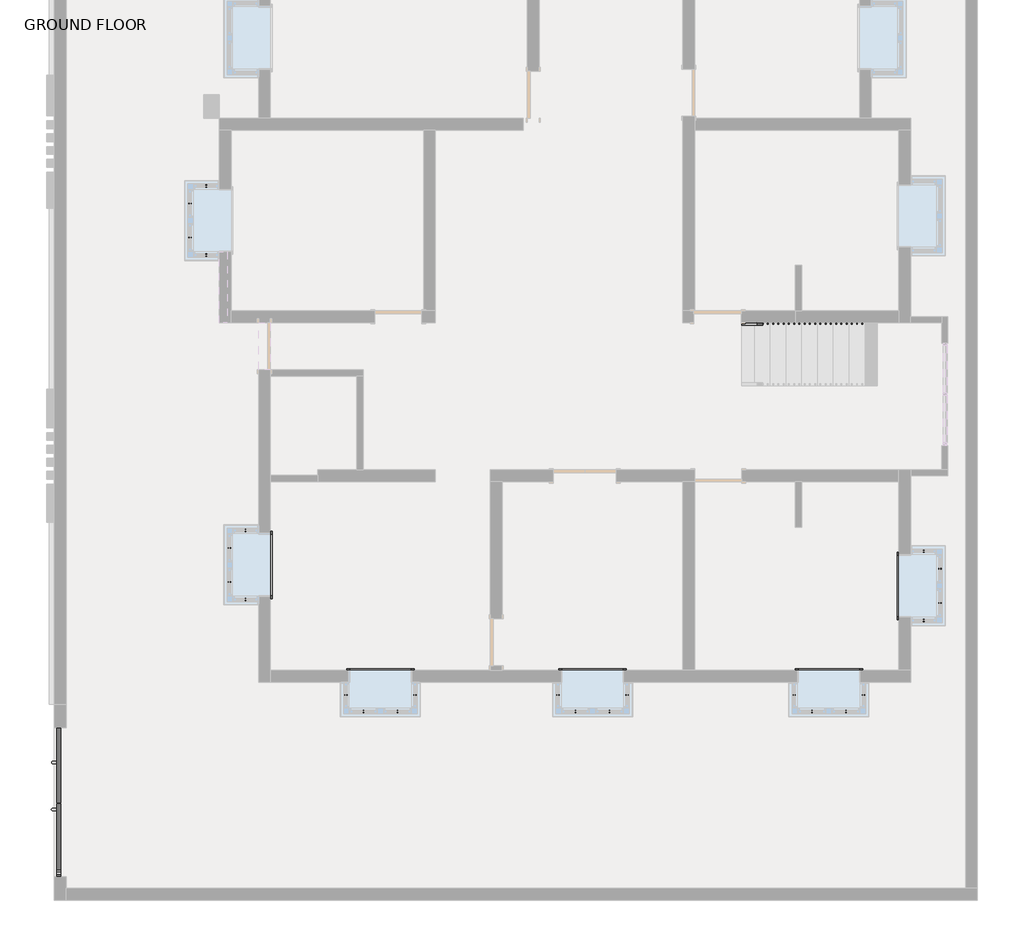
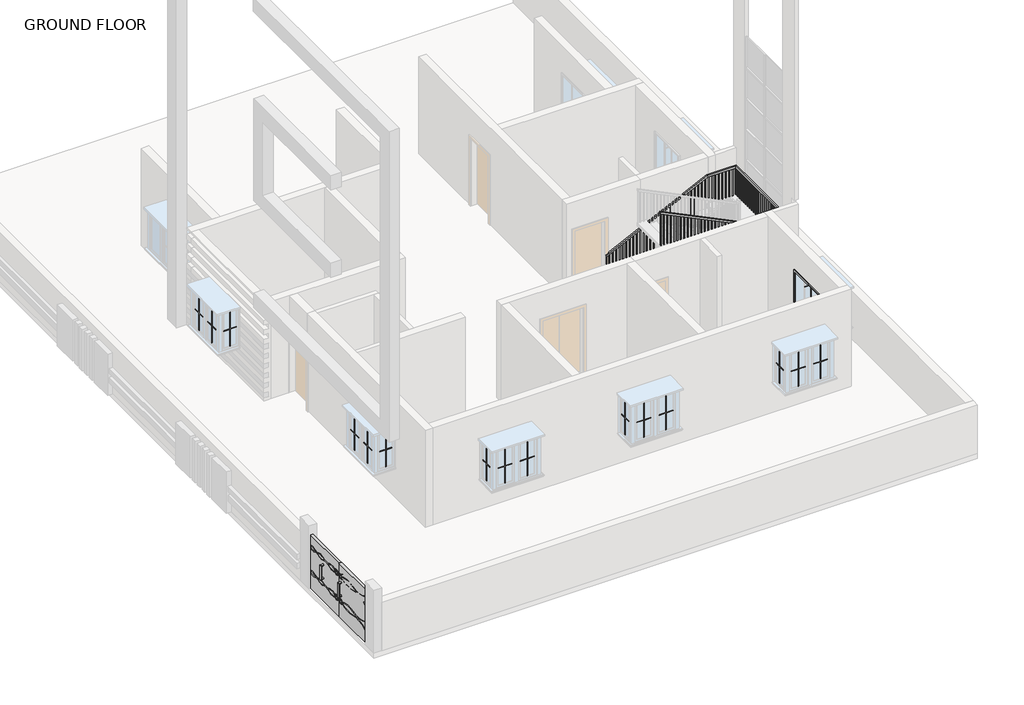
# One storey, part 4 of 5: 30 proxies, 1 railing.
"""IFC4 building model written with IfcOpenShell, lengths in millimetres."""

from ifc_helpers import new_model, si_unit, frame, origin, place, context, project, spatial, polyline, outline, extrude, faceted_brep, transform, mapped, element, save
from components import generic_models_a1fe0e04, muntin_pattern_2x2_muntin_pattern_2x2_4aee108e, muntin_pattern_2x2_muntin_pattern_2x2_f03ab90d, muntin_pattern_2x2_muntin_pattern_2x2_eb08c668, trim_window_interior_flat_picture_frame_ace0ae79

model = new_model("IFC4")

# Units and contexts
model_context = context("Model", 3, world=origin())
ifc_project = project(units=[si_unit("LENGTHUNIT", "METRE", prefix="MILLI")], contexts=[model_context])

# Site, building, storey
site = spatial("IfcSite", under=ifc_project)
building = spatial("IfcBuilding", under=site)
storey = spatial("IfcBuildingStorey", under=building, Name="GROUND FLOOR", Elevation=0.0)

# Proxies
placement = place(None, origin())
generic_models_shape = generic_models_a1fe0e04(model_context)
element("IfcBuildingElementProxy", 1, Name="Generic Models", at=placement, inside=storey, context=model_context, shape_type="MappedRepresentation", body=[
    mapped(generic_models_shape, transform((-10087.5827664, -9094.4684552, 0.0), x_axis=(0.0, -1.0, 0.0), y_axis=(1.0, 0.0, 0.0), z_axis=(0.0, 0.0, 1.0))),
])
muntin_pattern_2x2_muntin_pattern_2x2_shape = muntin_pattern_2x2_muntin_pattern_2x2_4aee108e(model_context)
element("IfcBuildingElementProxy", 2, Name="Muntin Pattern_2x2 : Muntin Pattern_2x2", ObjectType="Muntin Pattern_2x2 : Muntin Pattern_2x2", at=placement, inside=storey, context=model_context, shape_type="MappedRepresentation", body=[
    mapped(muntin_pattern_2x2_muntin_pattern_2x2_shape, transform((-7576.6665084, 1871.733346, 1035.05), x_axis=(0.0, 1.0, 0.0), y_axis=(-1.0, 0.0, 0.0), z_axis=(0.0, 0.0, 1.0))),
])
element("IfcBuildingElementProxy", 3, Name="Muntin Pattern_2x2 : Muntin Pattern_2x2", ObjectType="Muntin Pattern_2x2 : Muntin Pattern_2x2", at=placement, inside=storey, context=model_context, shape_type="MappedRepresentation", body=[
    mapped(muntin_pattern_2x2_muntin_pattern_2x2_shape, transform((-3553.9415084, -7319.891654, 1035.05), x_axis=(-1.0, 0.0, 0.0), y_axis=(0.0, -1.0, 0.0), z_axis=(0.0, 0.0, 1.0))),
])
element("IfcBuildingElementProxy", 4, Name="Muntin Pattern_2x2 : Muntin Pattern_2x2", ObjectType="Muntin Pattern_2x2 : Muntin Pattern_2x2", at=placement, inside=storey, context=model_context, shape_type="MappedRepresentation", body=[
    mapped(muntin_pattern_2x2_muntin_pattern_2x2_shape, transform((5145.5584916, -7319.891654, 1035.05), x_axis=(-1.0, 0.0, 0.0), y_axis=(0.0, -1.0, 0.0), z_axis=(0.0, 0.0, 1.0))),
])
element("IfcBuildingElementProxy", 5, Name="Muntin Pattern_2x2 : Muntin Pattern_2x2", ObjectType="Muntin Pattern_2x2 : Muntin Pattern_2x2", at=placement, inside=storey, context=model_context, shape_type="MappedRepresentation", body=[
    mapped(muntin_pattern_2x2_muntin_pattern_2x2_shape, transform((560.8584916, -7319.891654, 1035.05), x_axis=(-1.0, 0.0, 0.0), y_axis=(0.0, -1.0, 0.0), z_axis=(0.0, 0.0, 1.0))),
])
element("IfcBuildingElementProxy", 6, Name="Muntin Pattern_2x2 : Muntin Pattern_2x2", ObjectType="Muntin Pattern_2x2 : Muntin Pattern_2x2", at=placement, inside=storey, context=model_context, shape_type="MappedRepresentation", body=[
    mapped(muntin_pattern_2x2_muntin_pattern_2x2_shape, transform((-6814.6665084, -4808.466654, 1035.05), x_axis=(0.0, 1.0, 0.0), y_axis=(-1.0, 0.0, 0.0), z_axis=(0.0, 0.0, 1.0))),
])
element("IfcBuildingElementProxy", 7, Name="Muntin Pattern_2x2 : Muntin Pattern_2x2", ObjectType="Muntin Pattern_2x2 : Muntin Pattern_2x2", at=placement, inside=storey, context=model_context, shape_type="MappedRepresentation", body=[
    mapped(muntin_pattern_2x2_muntin_pattern_2x2_shape, transform((6971.1834916, -4554.466654, 1035.05), x_axis=(0.0, -1.0, 0.0), y_axis=(1.0, 0.0, 0.0), z_axis=(0.0, 0.0, 1.0))),
])
muntin_pattern_2x2_muntin_pattern_2x2_2_shape = muntin_pattern_2x2_muntin_pattern_2x2_f03ab90d(model_context)
element("IfcBuildingElementProxy", 8, Name="Muntin Pattern_2x2 : Muntin Pattern_2x2", ObjectType="Muntin Pattern_2x2 : Muntin Pattern_2x2", at=placement, inside=storey, context=model_context, shape_type="MappedRepresentation", body=[
    mapped(muntin_pattern_2x2_muntin_pattern_2x2_2_shape, transform((-7262.3415084, 1532.008346, 1035.05), x_axis=(1.0, 0.0, 0.0), y_axis=(0.0, 1.0, 0.0), z_axis=(0.0, 0.0, 1.0))),
])
element("IfcBuildingElementProxy", 9, Name="Muntin Pattern_2x2 : Muntin Pattern_2x2", ObjectType="Muntin Pattern_2x2 : Muntin Pattern_2x2", at=placement, inside=storey, context=model_context, shape_type="MappedRepresentation", body=[
    mapped(muntin_pattern_2x2_muntin_pattern_2x2_2_shape, transform((-7262.3415084, 2871.858346, 1035.05), x_axis=(-1.0, 0.0, 0.0), y_axis=(0.0, -1.0, 0.0), z_axis=(0.0, 0.0, 1.0))),
])
element("IfcBuildingElementProxy", 10, Name="Muntin Pattern_2x2 : Muntin Pattern_2x2", ObjectType="Muntin Pattern_2x2 : Muntin Pattern_2x2", at=placement, inside=storey, context=model_context, shape_type="MappedRepresentation", body=[
    mapped(muntin_pattern_2x2_muntin_pattern_2x2_2_shape, transform((-3214.2165084, -7005.566654, 1035.05), x_axis=(0.0, 1.0, 0.0), y_axis=(-1.0, 0.0, 0.0), z_axis=(0.0, 0.0, 1.0))),
])
element("IfcBuildingElementProxy", 11, Name="Muntin Pattern_2x2 : Muntin Pattern_2x2", ObjectType="Muntin Pattern_2x2 : Muntin Pattern_2x2", at=placement, inside=storey, context=model_context, shape_type="MappedRepresentation", body=[
    mapped(muntin_pattern_2x2_muntin_pattern_2x2_2_shape, transform((-4554.0665084, -7005.566654, 1035.05), x_axis=(0.0, -1.0, 0.0), y_axis=(1.0, 0.0, 0.0), z_axis=(0.0, 0.0, 1.0))),
])
element("IfcBuildingElementProxy", 12, Name="Muntin Pattern_2x2 : Muntin Pattern_2x2", ObjectType="Muntin Pattern_2x2 : Muntin Pattern_2x2", at=placement, inside=storey, context=model_context, shape_type="MappedRepresentation", body=[
    mapped(muntin_pattern_2x2_muntin_pattern_2x2_2_shape, transform((5485.2834916, -7005.566654, 1035.05), x_axis=(0.0, 1.0, 0.0), y_axis=(-1.0, 0.0, 0.0), z_axis=(0.0, 0.0, 1.0))),
])
element("IfcBuildingElementProxy", 13, Name="Muntin Pattern_2x2 : Muntin Pattern_2x2", ObjectType="Muntin Pattern_2x2 : Muntin Pattern_2x2", at=placement, inside=storey, context=model_context, shape_type="MappedRepresentation", body=[
    mapped(muntin_pattern_2x2_muntin_pattern_2x2_2_shape, transform((4145.4334916, -7005.566654, 1035.05), x_axis=(0.0, -1.0, 0.0), y_axis=(1.0, 0.0, 0.0), z_axis=(0.0, 0.0, 1.0))),
])
element("IfcBuildingElementProxy", 14, Name="Muntin Pattern_2x2 : Muntin Pattern_2x2", ObjectType="Muntin Pattern_2x2 : Muntin Pattern_2x2", at=placement, inside=storey, context=model_context, shape_type="MappedRepresentation", body=[
    mapped(muntin_pattern_2x2_muntin_pattern_2x2_2_shape, transform((900.5834916, -7005.566654, 1035.05), x_axis=(0.0, 1.0, 0.0), y_axis=(-1.0, 0.0, 0.0), z_axis=(0.0, 0.0, 1.0))),
])
element("IfcBuildingElementProxy", 15, Name="Muntin Pattern_2x2 : Muntin Pattern_2x2", ObjectType="Muntin Pattern_2x2 : Muntin Pattern_2x2", at=placement, inside=storey, context=model_context, shape_type="MappedRepresentation", body=[
    mapped(muntin_pattern_2x2_muntin_pattern_2x2_2_shape, transform((-439.2665084, -7005.566654, 1035.05), x_axis=(0.0, -1.0, 0.0), y_axis=(1.0, 0.0, 0.0), z_axis=(0.0, 0.0, 1.0))),
])
element("IfcBuildingElementProxy", 16, Name="Muntin Pattern_2x2 : Muntin Pattern_2x2", ObjectType="Muntin Pattern_2x2 : Muntin Pattern_2x2", at=placement, inside=storey, context=model_context, shape_type="MappedRepresentation", body=[
    mapped(muntin_pattern_2x2_muntin_pattern_2x2_2_shape, transform((-6500.3415084, -5148.191654, 1035.05), x_axis=(1.0, 0.0, 0.0), y_axis=(0.0, 1.0, 0.0), z_axis=(0.0, 0.0, 1.0))),
])
element("IfcBuildingElementProxy", 17, Name="Muntin Pattern_2x2 : Muntin Pattern_2x2", ObjectType="Muntin Pattern_2x2 : Muntin Pattern_2x2", at=placement, inside=storey, context=model_context, shape_type="MappedRepresentation", body=[
    mapped(muntin_pattern_2x2_muntin_pattern_2x2_2_shape, transform((-6500.3415084, -3808.341654, 1035.05), x_axis=(-1.0, 0.0, 0.0), y_axis=(0.0, -1.0, 0.0), z_axis=(0.0, 0.0, 1.0))),
])
element("IfcBuildingElementProxy", 18, Name="Muntin Pattern_2x2 : Muntin Pattern_2x2", ObjectType="Muntin Pattern_2x2 : Muntin Pattern_2x2", at=placement, inside=storey, context=model_context, shape_type="MappedRepresentation", body=[
    mapped(muntin_pattern_2x2_muntin_pattern_2x2_2_shape, transform((6656.8584916, -4214.741654, 1035.05), x_axis=(-1.0, 0.0, 0.0), y_axis=(0.0, -1.0, 0.0), z_axis=(0.0, 0.0, 1.0))),
])
element("IfcBuildingElementProxy", 19, Name="Muntin Pattern_2x2 : Muntin Pattern_2x2", ObjectType="Muntin Pattern_2x2 : Muntin Pattern_2x2", at=placement, inside=storey, context=model_context, shape_type="MappedRepresentation", body=[
    mapped(muntin_pattern_2x2_muntin_pattern_2x2_2_shape, transform((6656.8584916, -5554.591654, 1035.05), x_axis=(1.0, 0.0, 0.0), y_axis=(0.0, 1.0, 0.0), z_axis=(0.0, 0.0, 1.0))),
])
muntin_pattern_2x2_muntin_pattern_2x2_3_shape = muntin_pattern_2x2_muntin_pattern_2x2_eb08c668(model_context)
element("IfcBuildingElementProxy", 20, Name="Muntin Pattern_2x2 : Muntin Pattern_2x2", ObjectType="Muntin Pattern_2x2 : Muntin Pattern_2x2", at=placement, inside=storey, context=model_context, shape_type="MappedRepresentation", body=[
    mapped(muntin_pattern_2x2_muntin_pattern_2x2_3_shape, transform((-7576.6665084, 2532.133346, 1035.05), x_axis=(0.0, -1.0, 0.0), y_axis=(1.0, 0.0, 0.0), z_axis=(0.0, 0.0, 1.0))),
])
element("IfcBuildingElementProxy", 21, Name="Muntin Pattern_2x2 : Muntin Pattern_2x2", ObjectType="Muntin Pattern_2x2 : Muntin Pattern_2x2", at=placement, inside=storey, context=model_context, shape_type="MappedRepresentation", body=[
    mapped(muntin_pattern_2x2_muntin_pattern_2x2_3_shape, transform((-4214.3415084, -7319.891654, 1035.05), x_axis=(1.0, 0.0, 0.0), y_axis=(0.0, 1.0, 0.0), z_axis=(0.0, 0.0, 1.0))),
])
element("IfcBuildingElementProxy", 22, Name="Muntin Pattern_2x2 : Muntin Pattern_2x2", ObjectType="Muntin Pattern_2x2 : Muntin Pattern_2x2", at=placement, inside=storey, context=model_context, shape_type="MappedRepresentation", body=[
    mapped(muntin_pattern_2x2_muntin_pattern_2x2_3_shape, transform((4485.1584916, -7319.891654, 1035.05), x_axis=(1.0, 0.0, 0.0), y_axis=(0.0, 1.0, 0.0), z_axis=(0.0, 0.0, 1.0))),
])
element("IfcBuildingElementProxy", 23, Name="Muntin Pattern_2x2 : Muntin Pattern_2x2", ObjectType="Muntin Pattern_2x2 : Muntin Pattern_2x2", at=placement, inside=storey, context=model_context, shape_type="MappedRepresentation", body=[
    mapped(muntin_pattern_2x2_muntin_pattern_2x2_3_shape, transform((-99.5415084, -7319.891654, 1035.05), x_axis=(1.0, 0.0, 0.0), y_axis=(0.0, 1.0, 0.0), z_axis=(0.0, 0.0, 1.0))),
])
element("IfcBuildingElementProxy", 24, Name="Muntin Pattern_2x2 : Muntin Pattern_2x2", ObjectType="Muntin Pattern_2x2 : Muntin Pattern_2x2", at=placement, inside=storey, context=model_context, shape_type="MappedRepresentation", body=[
    mapped(muntin_pattern_2x2_muntin_pattern_2x2_3_shape, transform((-6814.6665084, -4148.066654, 1035.05), x_axis=(0.0, -1.0, 0.0), y_axis=(1.0, 0.0, 0.0), z_axis=(0.0, 0.0, 1.0))),
])
element("IfcBuildingElementProxy", 25, Name="Muntin Pattern_2x2 : Muntin Pattern_2x2", ObjectType="Muntin Pattern_2x2 : Muntin Pattern_2x2", at=placement, inside=storey, context=model_context, shape_type="MappedRepresentation", body=[
    mapped(muntin_pattern_2x2_muntin_pattern_2x2_3_shape, transform((6971.1834916, -5214.866654, 1035.05), x_axis=(0.0, 1.0, 0.0), y_axis=(-1.0, 0.0, 0.0), z_axis=(0.0, 0.0, 1.0))),
])
trim_window_interior_flat_picture_frame_shape = trim_window_interior_flat_picture_frame_ace0ae79(model_context)
element("IfcBuildingElementProxy", 26, Name="Trim-Window-Interior-Flat : Picture Frame", ObjectType="Trim-Window-Interior-Flat : Picture Frame", at=placement, inside=storey, context=model_context, shape_type="MappedRepresentation", body=[
    mapped(trim_window_interior_flat_picture_frame_shape, transform((-3884.1415084, -6522.966654, 2184.4), x_axis=(-1.0, 0.0, 0.0), y_axis=(0.0, 0.0, 1.0), z_axis=(0.0, 1.0, 0.0))),
])
element("IfcBuildingElementProxy", 27, Name="Trim-Window-Interior-Flat : Picture Frame", ObjectType="Trim-Window-Interior-Flat : Picture Frame", at=placement, inside=storey, context=model_context, shape_type="MappedRepresentation", body=[
    mapped(trim_window_interior_flat_picture_frame_shape, transform((4815.3584916, -6522.966654, 2184.4), x_axis=(-1.0, 0.0, 0.0), y_axis=(0.0, 0.0, 1.0), z_axis=(0.0, 1.0, 0.0))),
])
element("IfcBuildingElementProxy", 28, Name="Trim-Window-Interior-Flat : Picture Frame", ObjectType="Trim-Window-Interior-Flat : Picture Frame", at=placement, inside=storey, context=model_context, shape_type="MappedRepresentation", body=[
    mapped(trim_window_interior_flat_picture_frame_shape, transform((230.6584916, -6522.966654, 2184.4), x_axis=(-1.0, 0.0, 0.0), y_axis=(0.0, 0.0, 1.0), z_axis=(0.0, 1.0, 0.0))),
])
element("IfcBuildingElementProxy", 29, Name="Trim-Window-Interior-Flat : Picture Frame", ObjectType="Trim-Window-Interior-Flat : Picture Frame", at=placement, inside=storey, context=model_context, shape_type="MappedRepresentation", body=[
    mapped(trim_window_interior_flat_picture_frame_shape, transform((-6017.7415084, -4478.266654, 2184.4), x_axis=(0.0, 1.0, 0.0), y_axis=(0.0, 0.0, 1.0), z_axis=(1.0, 0.0, 0.0))),
])
element("IfcBuildingElementProxy", 30, Name="Trim-Window-Interior-Flat : Picture Frame", ObjectType="Trim-Window-Interior-Flat : Picture Frame", at=placement, inside=storey, context=model_context, shape_type="MappedRepresentation", body=[
    mapped(trim_window_interior_flat_picture_frame_shape, transform((6174.2584916, -4884.666654, 2184.4), x_axis=(0.0, -1.0, 0.0), y_axis=(0.0, 0.0, 1.0), z_axis=(-1.0, 0.0, 0.0))),
])

# Railing
element("IfcRailing", 31, ObjectType="Handrail - Rectangular", at=placement, inside=storey, context=model_context, shape_type="SolidModel", body=[
    faceted_brep([(3126.2584916, 220.733346, 1059.8727273), (3126.2584916, 220.733346, 1003.3956113), (3126.2584916, 169.933346, 1003.3956113), (3126.2584916, 169.933346, 1059.8727273), (6120.7829507, 220.733346, 2514.6), (6132.4691705, 220.733346, 2463.8), (6132.4691705, 169.933346, 2463.8), (6120.7829507, 169.933346, 2514.6), (7009.1350459, 220.733346, 2514.6), (7009.1350459, 220.733346, 2463.8), (6958.3350459, 169.933346, 2463.8), (6958.3350459, 169.933346, 2514.6), (7009.1350459, -2636.766654, 2514.6), (7009.1350459, -2636.766654, 2463.8), (6958.3350459, -2585.966654, 2463.8), (6958.3350459, -2585.966654, 2514.6), (6420.2353966, -2636.766654, 2514.6), (6408.5491768, -2636.766654, 2463.8), (6408.5491768, -2585.966654, 2463.8), (6420.2353966, -2585.966654, 2514.6), (3126.2584916, -2636.766654, 4114.8), (3126.2584916, -2585.966654, 4114.8), (3126.2584916, -2585.966654, 4058.322884), (3126.2584916, -2636.766654, 4058.322884)], [[[0, 1, 2, 3]], [[1, 0, 4, 5]], [[2, 1, 5, 6]], [[3, 2, 6, 7]], [[0, 3, 7, 4]], [[5, 4, 8, 9]], [[6, 5, 9, 10]], [[7, 6, 10, 11]], [[4, 7, 11, 8]], [[9, 8, 12, 13]], [[10, 9, 13, 14]], [[11, 10, 14, 15]], [[8, 11, 15, 12]], [[13, 12, 16, 17]], [[14, 13, 17, 18]], [[15, 14, 18, 19]], [[12, 15, 19, 16]], [[20, 21, 22, 23]], [[17, 16, 20, 23]], [[18, 17, 23, 22]], [[19, 18, 22, 21]], [[16, 19, 21, 20]]]),
    extrude(outline(polyline([(4015.2077556, 3215.0100459), (3054.9272727, 3215.0100459), (3054.9272727, 3234.0600459), (4005.9533465, 3234.0600459), (4015.2077556, 3215.0100459)])), frame((0.0, -2620.891654, 0.0), z_axis=(0.0, 1.0, 0.0), x_axis=(0.0, 0.0, 1.0)), (0.0, 0.0, 1.0), 19.05),
    extrude(outline(polyline([(3965.8509068, 3316.6100459), (3054.9272727, 3316.6100459), (3054.9272727, 3335.6600459), (3956.5964977, 3335.6600459), (3965.8509068, 3316.6100459)])), frame((0.0, -2620.891654, 0.0), z_axis=(0.0, 1.0, 0.0), x_axis=(0.0, 0.0, 1.0)), (0.0, 0.0, 1.0), 19.05),
    extrude(outline(polyline([(3916.494058, 3418.2100459), (2909.4545455, 3418.2100459), (2909.4545455, 3437.2600459), (3907.2396489, 3437.2600459), (3916.494058, 3418.2100459)])), frame((0.0, -2620.891654, 0.0), z_axis=(0.0, 1.0, 0.0), x_axis=(0.0, 0.0, 1.0)), (0.0, 0.0, 1.0), 19.05),
    extrude(outline(polyline([(3867.1372093, 3519.8100459), (2909.4545455, 3519.8100459), (2909.4545455, 3538.8600459), (3857.8828001, 3538.8600459), (3867.1372093, 3519.8100459)])), frame((0.0, -2620.891654, 0.0), z_axis=(0.0, 1.0, 0.0), x_axis=(0.0, 0.0, 1.0)), (0.0, 0.0, 1.0), 19.05),
    extrude(outline(polyline([(3817.7803605, 3621.4100459), (2909.4545455, 3621.4100459), (2909.4545455, 3640.4600459), (3808.5259513, 3640.4600459), (3817.7803605, 3621.4100459)])), frame((0.0, -2620.891654, 0.0), z_axis=(0.0, 1.0, 0.0), x_axis=(0.0, 0.0, 1.0)), (0.0, 0.0, 1.0), 19.05),
    extrude(outline(polyline([(3768.4235117, 3723.0100459), (2763.9818182, 3723.0100459), (2763.9818182, 3742.0600459), (3759.1691025, 3742.0600459), (3768.4235117, 3723.0100459)])), frame((0.0, -2620.891654, 0.0), z_axis=(0.0, 1.0, 0.0), x_axis=(0.0, 0.0, 1.0)), (0.0, 0.0, 1.0), 19.05),
    extrude(outline(polyline([(3719.0666629, 3824.6100459), (2763.9818182, 3824.6100459), (2763.9818182, 3843.6600459), (3709.8122538, 3843.6600459), (3719.0666629, 3824.6100459)])), frame((0.0, -2620.891654, 0.0), z_axis=(0.0, 1.0, 0.0), x_axis=(0.0, 0.0, 1.0)), (0.0, 0.0, 1.0), 19.05),
    extrude(outline(polyline([(3669.7098141, 3926.2100459), (2763.9818182, 3926.2100459), (2763.9818182, 3945.2600459), (3660.455405, 3945.2600459), (3669.7098141, 3926.2100459)])), frame((0.0, -2620.891654, 0.0), z_axis=(0.0, 1.0, 0.0), x_axis=(0.0, 0.0, 1.0)), (0.0, 0.0, 1.0), 19.05),
    extrude(outline(polyline([(3620.3529653, 4027.8100459), (2618.5090909, 4027.8100459), (2618.5090909, 4046.8600459), (3611.0985562, 4046.8600459), (3620.3529653, 4027.8100459)])), frame((0.0, -2620.891654, 0.0), z_axis=(0.0, 1.0, 0.0), x_axis=(0.0, 0.0, 1.0)), (0.0, 0.0, 1.0), 19.05),
    extrude(outline(polyline([(3570.9961165, 4129.4100459), (2618.5090909, 4129.4100459), (2618.5090909, 4148.4600459), (3561.7417074, 4148.4600459), (3570.9961165, 4129.4100459)])), frame((0.0, -2620.891654, 0.0), z_axis=(0.0, 1.0, 0.0), x_axis=(0.0, 0.0, 1.0)), (0.0, 0.0, 1.0), 19.05),
    extrude(outline(polyline([(3521.6392678, 4231.0100459), (2618.5090909, 4231.0100459), (2618.5090909, 4250.0600459), (3512.3848586, 4250.0600459), (3521.6392678, 4231.0100459)])), frame((0.0, -2620.891654, 0.0), z_axis=(0.0, 1.0, 0.0), x_axis=(0.0, 0.0, 1.0)), (0.0, 0.0, 1.0), 19.05),
    extrude(outline(polyline([(3472.282419, 4332.6100459), (2473.0363636, 4332.6100459), (2473.0363636, 4351.6600459), (3463.0280098, 4351.6600459), (3472.282419, 4332.6100459)])), frame((0.0, -2620.891654, 0.0), z_axis=(0.0, 1.0, 0.0), x_axis=(0.0, 0.0, 1.0)), (0.0, 0.0, 1.0), 19.05),
    extrude(outline(polyline([(3422.9255702, 4434.2100459), (2473.0363636, 4434.2100459), (2473.0363636, 4453.2600459), (3413.671161, 4453.2600459), (3422.9255702, 4434.2100459)])), frame((0.0, -2620.891654, 0.0), z_axis=(0.0, 1.0, 0.0), x_axis=(0.0, 0.0, 1.0)), (0.0, 0.0, 1.0), 19.05),
    extrude(outline(polyline([(3373.5687214, 4535.8100459), (2473.0363636, 4535.8100459), (2473.0363636, 4554.8600459), (3364.3143123, 4554.8600459), (3373.5687214, 4535.8100459)])), frame((0.0, -2620.891654, 0.0), z_axis=(0.0, 1.0, 0.0), x_axis=(0.0, 0.0, 1.0)), (0.0, 0.0, 1.0), 19.05),
    extrude(outline(polyline([(3324.2118726, 4637.4100459), (2327.5636364, 4637.4100459), (2327.5636364, 4656.4600459), (3314.9574635, 4656.4600459), (3324.2118726, 4637.4100459)])), frame((0.0, -2620.891654, 0.0), z_axis=(0.0, 1.0, 0.0), x_axis=(0.0, 0.0, 1.0)), (0.0, 0.0, 1.0), 19.05),
    extrude(outline(polyline([(3274.8550238, 4739.0100459), (2327.5636364, 4739.0100459), (2327.5636364, 4758.0600459), (3265.6006147, 4758.0600459), (3274.8550238, 4739.0100459)])), frame((0.0, -2620.891654, 0.0), z_axis=(0.0, 1.0, 0.0), x_axis=(0.0, 0.0, 1.0)), (0.0, 0.0, 1.0), 19.05),
    extrude(outline(polyline([(3225.4981751, 4840.6100459), (2327.5636364, 4840.6100459), (2327.5636364, 4859.6600459), (3216.2437659, 4859.6600459), (3225.4981751, 4840.6100459)])), frame((0.0, -2620.891654, 0.0), z_axis=(0.0, 1.0, 0.0), x_axis=(0.0, 0.0, 1.0)), (0.0, 0.0, 1.0), 19.05),
    extrude(outline(polyline([(3176.1413263, 4942.2100459), (2182.0909091, 4942.2100459), (2182.0909091, 4961.2600459), (3166.8869171, 4961.2600459), (3176.1413263, 4942.2100459)])), frame((0.0, -2620.891654, 0.0), z_axis=(0.0, 1.0, 0.0), x_axis=(0.0, 0.0, 1.0)), (0.0, 0.0, 1.0), 19.05),
    extrude(outline(polyline([(3126.7844775, 5043.8100459), (2182.0909091, 5043.8100459), (2182.0909091, 5062.8600459), (3117.5300683, 5062.8600459), (3126.7844775, 5043.8100459)])), frame((0.0, -2620.891654, 0.0), z_axis=(0.0, 1.0, 0.0), x_axis=(0.0, 0.0, 1.0)), (0.0, 0.0, 1.0), 19.05),
    extrude(outline(polyline([(3077.4276287, 5145.4100459), (2182.0909091, 5145.4100459), (2182.0909091, 5164.4600459), (3068.1732196, 5164.4600459), (3077.4276287, 5145.4100459)])), frame((0.0, -2620.891654, 0.0), z_axis=(0.0, 1.0, 0.0), x_axis=(0.0, 0.0, 1.0)), (0.0, 0.0, 1.0), 19.05),
    extrude(outline(polyline([(3028.0707799, 5247.0100459), (2036.6181818, 5247.0100459), (2036.6181818, 5266.0600459), (3018.8163708, 5266.0600459), (3028.0707799, 5247.0100459)])), frame((0.0, -2620.891654, 0.0), z_axis=(0.0, 1.0, 0.0), x_axis=(0.0, 0.0, 1.0)), (0.0, 0.0, 1.0), 19.05),
    extrude(outline(polyline([(2978.7139311, 5348.6100459), (2036.6181818, 5348.6100459), (2036.6181818, 5367.6600459), (2969.459522, 5367.6600459), (2978.7139311, 5348.6100459)])), frame((0.0, -2620.891654, 0.0), z_axis=(0.0, 1.0, 0.0), x_axis=(0.0, 0.0, 1.0)), (0.0, 0.0, 1.0), 19.05),
    extrude(outline(polyline([(2929.3570823, 5450.2100459), (2036.6181818, 5450.2100459), (2036.6181818, 5469.2600459), (2920.1026732, 5469.2600459), (2929.3570823, 5450.2100459)])), frame((0.0, -2620.891654, 0.0), z_axis=(0.0, 1.0, 0.0), x_axis=(0.0, 0.0, 1.0)), (0.0, 0.0, 1.0), 19.05),
    extrude(outline(polyline([(2880.0002336, 5551.8100459), (1891.1454545, 5551.8100459), (1891.1454545, 5570.8600459), (2870.7458244, 5570.8600459), (2880.0002336, 5551.8100459)])), frame((0.0, -2620.891654, 0.0), z_axis=(0.0, 1.0, 0.0), x_axis=(0.0, 0.0, 1.0)), (0.0, 0.0, 1.0), 19.05),
    extrude(outline(polyline([(2830.6433848, 5653.4100459), (1891.1454545, 5653.4100459), (1891.1454545, 5672.4600459), (2821.3889756, 5672.4600459), (2830.6433848, 5653.4100459)])), frame((0.0, -2620.891654, 0.0), z_axis=(0.0, 1.0, 0.0), x_axis=(0.0, 0.0, 1.0)), (0.0, 0.0, 1.0), 19.05),
    extrude(outline(polyline([(2781.286536, 5755.0100459), (1891.1454545, 5755.0100459), (1891.1454545, 5774.0600459), (2772.0321268, 5774.0600459), (2781.286536, 5755.0100459)])), frame((0.0, -2620.891654, 0.0), z_axis=(0.0, 1.0, 0.0), x_axis=(0.0, 0.0, 1.0)), (0.0, 0.0, 1.0), 19.05),
    extrude(outline(polyline([(2731.9296872, 5856.6100459), (1745.6727273, 5856.6100459), (1745.6727273, 5875.6600459), (2722.6752781, 5875.6600459), (2731.9296872, 5856.6100459)])), frame((0.0, -2620.891654, 0.0), z_axis=(0.0, 1.0, 0.0), x_axis=(0.0, 0.0, 1.0)), (0.0, 0.0, 1.0), 19.05),
    extrude(outline(polyline([(2682.5728384, 5958.2100459), (1745.6727273, 5958.2100459), (1745.6727273, 5977.2600459), (2673.3184293, 5977.2600459), (2682.5728384, 5958.2100459)])), frame((0.0, -2620.891654, 0.0), z_axis=(0.0, 1.0, 0.0), x_axis=(0.0, 0.0, 1.0)), (0.0, 0.0, 1.0), 19.05),
    extrude(outline(polyline([(2633.2159896, 6059.8100459), (1745.6727273, 6059.8100459), (1745.6727273, 6078.8600459), (2623.9615805, 6078.8600459), (2633.2159896, 6059.8100459)])), frame((0.0, -2620.891654, 0.0), z_axis=(0.0, 1.0, 0.0), x_axis=(0.0, 0.0, 1.0)), (0.0, 0.0, 1.0), 19.05),
    extrude(outline(polyline([(2583.8591409, 6161.4100459), (1600.2, 6161.4100459), (1600.2, 6180.4600459), (2574.6047317, 6180.4600459), (2583.8591409, 6161.4100459)])), frame((0.0, -2620.891654, 0.0), z_axis=(0.0, 1.0, 0.0), x_axis=(0.0, 0.0, 1.0)), (0.0, 0.0, 1.0), 19.05),
    extrude(outline(polyline([(2534.5022921, 6263.0100459), (1600.2, 6263.0100459), (1600.2, 6282.0600459), (2525.2478829, 6282.0600459), (2534.5022921, 6263.0100459)])), frame((0.0, -2620.891654, 0.0), z_axis=(0.0, 1.0, 0.0), x_axis=(0.0, 0.0, 1.0)), (0.0, 0.0, 1.0), 19.05),
    extrude(outline(polyline([(2485.1454433, 6364.6100459), (1600.2, 6364.6100459), (1600.2, 6383.6600459), (2475.8910341, 6383.6600459), (2485.1454433, 6364.6100459)])), frame((0.0, -2620.891654, 0.0), z_axis=(0.0, 1.0, 0.0), x_axis=(0.0, 0.0, 1.0)), (0.0, 0.0, 1.0), 19.05),
    extrude(outline(polyline([(6485.2600459, -2620.891654), (6466.2100459, -2620.891654), (6466.2100459, -2601.841654), (6485.2600459, -2601.841654), (6485.2600459, -2620.891654)])), frame((0.0, 0.0, 1600.2), z_axis=(0.0, 0.0, 1.0), x_axis=(1.0, 0.0, 0.0)), (0.0, 0.0, 1.0), 863.6),
    extrude(outline(polyline([(6586.8600459, -2620.891654), (6567.8100459, -2620.891654), (6567.8100459, -2601.841654), (6586.8600459, -2601.841654), (6586.8600459, -2620.891654)])), frame((0.0, 0.0, 1600.2), z_axis=(0.0, 0.0, 1.0), x_axis=(1.0, 0.0, 0.0)), (0.0, 0.0, 1.0), 863.6),
    extrude(outline(polyline([(6688.4600459, -2620.891654), (6669.4100459, -2620.891654), (6669.4100459, -2601.841654), (6688.4600459, -2601.841654), (6688.4600459, -2620.891654)])), frame((0.0, 0.0, 1600.2), z_axis=(0.0, 0.0, 1.0), x_axis=(1.0, 0.0, 0.0)), (0.0, 0.0, 1.0), 863.6),
    extrude(outline(polyline([(6790.0600459, -2620.891654), (6771.0100459, -2620.891654), (6771.0100459, -2601.841654), (6790.0600459, -2601.841654), (6790.0600459, -2620.891654)])), frame((0.0, 0.0, 1600.2), z_axis=(0.0, 0.0, 1.0), x_axis=(1.0, 0.0, 0.0)), (0.0, 0.0, 1.0), 863.6),
    extrude(outline(polyline([(6891.6600459, -2620.891654), (6872.6100459, -2620.891654), (6872.6100459, -2601.841654), (6891.6600459, -2601.841654), (6891.6600459, -2620.891654)])), frame((0.0, 0.0, 1600.2), z_axis=(0.0, 0.0, 1.0), x_axis=(1.0, 0.0, 0.0)), (0.0, 0.0, 1.0), 863.6),
    extrude(outline(polyline([(6993.2600459, -2538.341654), (6993.2600459, -2557.391654), (6974.2100459, -2557.391654), (6974.2100459, -2538.341654), (6993.2600459, -2538.341654)])), frame((0.0, 0.0, 1600.2), z_axis=(0.0, 0.0, 1.0), x_axis=(1.0, 0.0, 0.0)), (0.0, 0.0, 1.0), 863.6),
    extrude(outline(polyline([(6993.2600459, -2436.741654), (6993.2600459, -2455.791654), (6974.2100459, -2455.791654), (6974.2100459, -2436.741654), (6993.2600459, -2436.741654)])), frame((0.0, 0.0, 1600.2), z_axis=(0.0, 0.0, 1.0), x_axis=(1.0, 0.0, 0.0)), (0.0, 0.0, 1.0), 863.6),
    extrude(outline(polyline([(6993.2600459, -2335.141654), (6993.2600459, -2354.191654), (6974.2100459, -2354.191654), (6974.2100459, -2335.141654), (6993.2600459, -2335.141654)])), frame((0.0, 0.0, 1600.2), z_axis=(0.0, 0.0, 1.0), x_axis=(1.0, 0.0, 0.0)), (0.0, 0.0, 1.0), 863.6),
    extrude(outline(polyline([(6993.2600459, -2233.541654), (6993.2600459, -2252.591654), (6974.2100459, -2252.591654), (6974.2100459, -2233.541654), (6993.2600459, -2233.541654)])), frame((0.0, 0.0, 1600.2), z_axis=(0.0, 0.0, 1.0), x_axis=(1.0, 0.0, 0.0)), (0.0, 0.0, 1.0), 863.6),
    extrude(outline(polyline([(6993.2600459, -2131.941654), (6993.2600459, -2150.991654), (6974.2100459, -2150.991654), (6974.2100459, -2131.941654), (6993.2600459, -2131.941654)])), frame((0.0, 0.0, 1600.2), z_axis=(0.0, 0.0, 1.0), x_axis=(1.0, 0.0, 0.0)), (0.0, 0.0, 1.0), 863.6),
    extrude(outline(polyline([(6993.2600459, -2030.341654), (6993.2600459, -2049.391654), (6974.2100459, -2049.391654), (6974.2100459, -2030.341654), (6993.2600459, -2030.341654)])), frame((0.0, 0.0, 1600.2), z_axis=(0.0, 0.0, 1.0), x_axis=(1.0, 0.0, 0.0)), (0.0, 0.0, 1.0), 863.6),
    extrude(outline(polyline([(6993.2600459, -1928.741654), (6993.2600459, -1947.791654), (6974.2100459, -1947.791654), (6974.2100459, -1928.741654), (6993.2600459, -1928.741654)])), frame((0.0, 0.0, 1600.2), z_axis=(0.0, 0.0, 1.0), x_axis=(1.0, 0.0, 0.0)), (0.0, 0.0, 1.0), 863.6),
    extrude(outline(polyline([(6993.2600459, -1827.141654), (6993.2600459, -1846.191654), (6974.2100459, -1846.191654), (6974.2100459, -1827.141654), (6993.2600459, -1827.141654)])), frame((0.0, 0.0, 1600.2), z_axis=(0.0, 0.0, 1.0), x_axis=(1.0, 0.0, 0.0)), (0.0, 0.0, 1.0), 863.6),
    extrude(outline(polyline([(6993.2600459, -1725.541654), (6993.2600459, -1744.591654), (6974.2100459, -1744.591654), (6974.2100459, -1725.541654), (6993.2600459, -1725.541654)])), frame((0.0, 0.0, 1600.2), z_axis=(0.0, 0.0, 1.0), x_axis=(1.0, 0.0, 0.0)), (0.0, 0.0, 1.0), 863.6),
    extrude(outline(polyline([(6993.2600459, -1623.941654), (6993.2600459, -1642.991654), (6974.2100459, -1642.991654), (6974.2100459, -1623.941654), (6993.2600459, -1623.941654)])), frame((0.0, 0.0, 1600.2), z_axis=(0.0, 0.0, 1.0), x_axis=(1.0, 0.0, 0.0)), (0.0, 0.0, 1.0), 863.6),
    extrude(outline(polyline([(6993.2600459, -1522.341654), (6993.2600459, -1541.391654), (6974.2100459, -1541.391654), (6974.2100459, -1522.341654), (6993.2600459, -1522.341654)])), frame((0.0, 0.0, 1600.2), z_axis=(0.0, 0.0, 1.0), x_axis=(1.0, 0.0, 0.0)), (0.0, 0.0, 1.0), 863.6),
    extrude(outline(polyline([(6993.2600459, -1420.741654), (6993.2600459, -1439.791654), (6974.2100459, -1439.791654), (6974.2100459, -1420.741654), (6993.2600459, -1420.741654)])), frame((0.0, 0.0, 1600.2), z_axis=(0.0, 0.0, 1.0), x_axis=(1.0, 0.0, 0.0)), (0.0, 0.0, 1.0), 863.6),
    extrude(outline(polyline([(6993.2600459, -1319.141654), (6993.2600459, -1338.191654), (6974.2100459, -1338.191654), (6974.2100459, -1319.141654), (6993.2600459, -1319.141654)])), frame((0.0, 0.0, 1600.2), z_axis=(0.0, 0.0, 1.0), x_axis=(1.0, 0.0, 0.0)), (0.0, 0.0, 1.0), 863.6),
    extrude(outline(polyline([(6993.2600459, -1217.541654), (6993.2600459, -1236.591654), (6974.2100459, -1236.591654), (6974.2100459, -1217.541654), (6993.2600459, -1217.541654)])), frame((0.0, 0.0, 1600.2), z_axis=(0.0, 0.0, 1.0), x_axis=(1.0, 0.0, 0.0)), (0.0, 0.0, 1.0), 863.6),
    extrude(outline(polyline([(6993.2600459, -1115.941654), (6993.2600459, -1134.991654), (6974.2100459, -1134.991654), (6974.2100459, -1115.941654), (6993.2600459, -1115.941654)])), frame((0.0, 0.0, 1600.2), z_axis=(0.0, 0.0, 1.0), x_axis=(1.0, 0.0, 0.0)), (0.0, 0.0, 1.0), 863.6),
    extrude(outline(polyline([(6993.2600459, -1014.341654), (6993.2600459, -1033.391654), (6974.2100459, -1033.391654), (6974.2100459, -1014.341654), (6993.2600459, -1014.341654)])), frame((0.0, 0.0, 1600.2), z_axis=(0.0, 0.0, 1.0), x_axis=(1.0, 0.0, 0.0)), (0.0, 0.0, 1.0), 863.6),
    extrude(outline(polyline([(6993.2600459, -912.741654), (6993.2600459, -931.791654), (6974.2100459, -931.791654), (6974.2100459, -912.741654), (6993.2600459, -912.741654)])), frame((0.0, 0.0, 1600.2), z_axis=(0.0, 0.0, 1.0), x_axis=(1.0, 0.0, 0.0)), (0.0, 0.0, 1.0), 863.6),
    extrude(outline(polyline([(6993.2600459, -811.141654), (6993.2600459, -830.191654), (6974.2100459, -830.191654), (6974.2100459, -811.141654), (6993.2600459, -811.141654)])), frame((0.0, 0.0, 1600.2), z_axis=(0.0, 0.0, 1.0), x_axis=(1.0, 0.0, 0.0)), (0.0, 0.0, 1.0), 863.6),
    extrude(outline(polyline([(6993.2600459, -709.541654), (6993.2600459, -728.591654), (6974.2100459, -728.591654), (6974.2100459, -709.541654), (6993.2600459, -709.541654)])), frame((0.0, 0.0, 1600.2), z_axis=(0.0, 0.0, 1.0), x_axis=(1.0, 0.0, 0.0)), (0.0, 0.0, 1.0), 863.6),
    extrude(outline(polyline([(6993.2600459, -607.941654), (6993.2600459, -626.991654), (6974.2100459, -626.991654), (6974.2100459, -607.941654), (6993.2600459, -607.941654)])), frame((0.0, 0.0, 1600.2), z_axis=(0.0, 0.0, 1.0), x_axis=(1.0, 0.0, 0.0)), (0.0, 0.0, 1.0), 863.6),
    extrude(outline(polyline([(6993.2600459, -506.341654), (6993.2600459, -525.391654), (6974.2100459, -525.391654), (6974.2100459, -506.341654), (6993.2600459, -506.341654)])), frame((0.0, 0.0, 1600.2), z_axis=(0.0, 0.0, 1.0), x_axis=(1.0, 0.0, 0.0)), (0.0, 0.0, 1.0), 863.6),
    extrude(outline(polyline([(6993.2600459, -404.741654), (6993.2600459, -423.791654), (6974.2100459, -423.791654), (6974.2100459, -404.741654), (6993.2600459, -404.741654)])), frame((0.0, 0.0, 1600.2), z_axis=(0.0, 0.0, 1.0), x_axis=(1.0, 0.0, 0.0)), (0.0, 0.0, 1.0), 863.6),
    extrude(outline(polyline([(6993.2600459, -303.141654), (6993.2600459, -322.191654), (6974.2100459, -322.191654), (6974.2100459, -303.141654), (6993.2600459, -303.141654)])), frame((0.0, 0.0, 1600.2), z_axis=(0.0, 0.0, 1.0), x_axis=(1.0, 0.0, 0.0)), (0.0, 0.0, 1.0), 863.6),
    extrude(outline(polyline([(6993.2600459, -201.541654), (6993.2600459, -220.591654), (6974.2100459, -220.591654), (6974.2100459, -201.541654), (6993.2600459, -201.541654)])), frame((0.0, 0.0, 1600.2), z_axis=(0.0, 0.0, 1.0), x_axis=(1.0, 0.0, 0.0)), (0.0, 0.0, 1.0), 863.6),
    extrude(outline(polyline([(6993.2600459, -99.941654), (6993.2600459, -118.991654), (6974.2100459, -118.991654), (6974.2100459, -99.941654), (6993.2600459, -99.941654)])), frame((0.0, 0.0, 1600.2), z_axis=(0.0, 0.0, 1.0), x_axis=(1.0, 0.0, 0.0)), (0.0, 0.0, 1.0), 863.6),
    extrude(outline(polyline([(6993.2600459, 1.658346), (6993.2600459, -17.391654), (6974.2100459, -17.391654), (6974.2100459, 1.658346), (6993.2600459, 1.658346)])), frame((0.0, 0.0, 1600.2), z_axis=(0.0, 0.0, 1.0), x_axis=(1.0, 0.0, 0.0)), (0.0, 0.0, 1.0), 863.6),
    extrude(outline(polyline([(6993.2600459, 103.258346), (6993.2600459, 84.208346), (6974.2100459, 84.208346), (6974.2100459, 103.258346), (6993.2600459, 103.258346)])), frame((0.0, 0.0, 1600.2), z_axis=(0.0, 0.0, 1.0), x_axis=(1.0, 0.0, 0.0)), (0.0, 0.0, 1.0), 863.6),
    extrude(outline(polyline([(6875.9334916, 204.858346), (6894.9834916, 204.858346), (6894.9834916, 185.808346), (6875.9334916, 185.808346), (6875.9334916, 204.858346)])), frame((0.0, 0.0, 1600.2), z_axis=(0.0, 0.0, 1.0), x_axis=(1.0, 0.0, 0.0)), (0.0, 0.0, 1.0), 863.6),
    extrude(outline(polyline([(6774.3334916, 204.858346), (6793.3834916, 204.858346), (6793.3834916, 185.808346), (6774.3334916, 185.808346), (6774.3334916, 204.858346)])), frame((0.0, 0.0, 1600.2), z_axis=(0.0, 0.0, 1.0), x_axis=(1.0, 0.0, 0.0)), (0.0, 0.0, 1.0), 863.6),
    extrude(outline(polyline([(6672.7334916, 204.858346), (6691.7834916, 204.858346), (6691.7834916, 185.808346), (6672.7334916, 185.808346), (6672.7334916, 204.858346)])), frame((0.0, 0.0, 1600.2), z_axis=(0.0, 0.0, 1.0), x_axis=(1.0, 0.0, 0.0)), (0.0, 0.0, 1.0), 863.6),
    extrude(outline(polyline([(6571.1334916, 204.858346), (6590.1834916, 204.858346), (6590.1834916, 185.808346), (6571.1334916, 185.808346), (6571.1334916, 204.858346)])), frame((0.0, 0.0, 1600.2), z_axis=(0.0, 0.0, 1.0), x_axis=(1.0, 0.0, 0.0)), (0.0, 0.0, 1.0), 863.6),
    extrude(outline(polyline([(6469.5334916, 204.858346), (6488.5834916, 204.858346), (6488.5834916, 185.808346), (6469.5334916, 185.808346), (6469.5334916, 204.858346)])), frame((0.0, 0.0, 1600.2), z_axis=(0.0, 0.0, 1.0), x_axis=(1.0, 0.0, 0.0)), (0.0, 0.0, 1.0), 863.6),
    extrude(outline(polyline([(6367.9334916, 204.858346), (6386.9834916, 204.858346), (6386.9834916, 185.808346), (6367.9334916, 185.808346), (6367.9334916, 204.858346)])), frame((0.0, 0.0, 1600.2), z_axis=(0.0, 0.0, 1.0), x_axis=(1.0, 0.0, 0.0)), (0.0, 0.0, 1.0), 863.6),
    extrude(outline(polyline([(6266.3334916, 204.858346), (6285.3834916, 204.858346), (6285.3834916, 185.808346), (6266.3334916, 185.808346), (6266.3334916, 204.858346)])), frame((0.0, 0.0, 1600.2), z_axis=(0.0, 0.0, 1.0), x_axis=(1.0, 0.0, 0.0)), (0.0, 0.0, 1.0), 863.6),
    extrude(outline(polyline([(6164.7334916, 204.858346), (6183.7834916, 204.858346), (6183.7834916, 185.808346), (6164.7334916, 185.808346), (6164.7334916, 204.858346)])), frame((0.0, 0.0, 1600.2), z_axis=(0.0, 0.0, 1.0), x_axis=(1.0, 0.0, 0.0)), (0.0, 0.0, 1.0), 863.6),
    extrude(outline(polyline([(2430.1170215, 6063.1334916), (1454.7272727, 6063.1334916), (1454.7272727, 6082.1834916), (2439.3714306, 6082.1834916), (2430.1170215, 6063.1334916)])), frame((0.0, 185.808346, 0.0), z_axis=(0.0, 1.0, 0.0), x_axis=(0.0, 0.0, 1.0)), (0.0, 0.0, 1.0), 19.05),
    extrude(outline(polyline([(2380.7601727, 5961.5334916), (1454.7272727, 5961.5334916), (1454.7272727, 5980.5834916), (2390.0145818, 5980.5834916), (2380.7601727, 5961.5334916)])), frame((0.0, 185.808346, 0.0), z_axis=(0.0, 1.0, 0.0), x_axis=(0.0, 0.0, 1.0)), (0.0, 0.0, 1.0), 19.05),
    extrude(outline(polyline([(2331.4033239, 5859.9334916), (1454.7272727, 5859.9334916), (1454.7272727, 5878.9834916), (2340.657733, 5878.9834916), (2331.4033239, 5859.9334916)])), frame((0.0, 185.808346, 0.0), z_axis=(0.0, 1.0, 0.0), x_axis=(0.0, 0.0, 1.0)), (0.0, 0.0, 1.0), 19.05),
    extrude(outline(polyline([(2282.0464751, 5758.3334916), (1309.2545455, 5758.3334916), (1309.2545455, 5777.3834916), (2291.3008843, 5777.3834916), (2282.0464751, 5758.3334916)])), frame((0.0, 185.808346, 0.0), z_axis=(0.0, 1.0, 0.0), x_axis=(0.0, 0.0, 1.0)), (0.0, 0.0, 1.0), 19.05),
    extrude(outline(polyline([(2232.6896263, 5656.7334916), (1309.2545455, 5656.7334916), (1309.2545455, 5675.7834916), (2241.9440355, 5675.7834916), (2232.6896263, 5656.7334916)])), frame((0.0, 185.808346, 0.0), z_axis=(0.0, 1.0, 0.0), x_axis=(0.0, 0.0, 1.0)), (0.0, 0.0, 1.0), 19.05),
    extrude(outline(polyline([(2183.3327775, 5555.1334916), (1309.2545455, 5555.1334916), (1309.2545455, 5574.1834916), (2192.5871867, 5574.1834916), (2183.3327775, 5555.1334916)])), frame((0.0, 185.808346, 0.0), z_axis=(0.0, 1.0, 0.0), x_axis=(0.0, 0.0, 1.0)), (0.0, 0.0, 1.0), 19.05),
    extrude(outline(polyline([(2133.9759288, 5453.5334916), (1163.7818182, 5453.5334916), (1163.7818182, 5472.5834916), (2143.2303379, 5472.5834916), (2133.9759288, 5453.5334916)])), frame((0.0, 185.808346, 0.0), z_axis=(0.0, 1.0, 0.0), x_axis=(0.0, 0.0, 1.0)), (0.0, 0.0, 1.0), 19.05),
    extrude(outline(polyline([(2084.61908, 5351.9334916), (1163.7818182, 5351.9334916), (1163.7818182, 5370.9834916), (2093.8734891, 5370.9834916), (2084.61908, 5351.9334916)])), frame((0.0, 185.808346, 0.0), z_axis=(0.0, 1.0, 0.0), x_axis=(0.0, 0.0, 1.0)), (0.0, 0.0, 1.0), 19.05),
    extrude(outline(polyline([(2035.2622312, 5250.3334916), (1163.7818182, 5250.3334916), (1163.7818182, 5269.3834916), (2044.5166403, 5269.3834916), (2035.2622312, 5250.3334916)])), frame((0.0, 185.808346, 0.0), z_axis=(0.0, 1.0, 0.0), x_axis=(0.0, 0.0, 1.0)), (0.0, 0.0, 1.0), 19.05),
    extrude(outline(polyline([(1985.9053824, 5148.7334916), (1018.3090909, 5148.7334916), (1018.3090909, 5167.7834916), (1995.1597915, 5167.7834916), (1985.9053824, 5148.7334916)])), frame((0.0, 185.808346, 0.0), z_axis=(0.0, 1.0, 0.0), x_axis=(0.0, 0.0, 1.0)), (0.0, 0.0, 1.0), 19.05),
    extrude(outline(polyline([(1936.5485336, 5047.1334916), (1018.3090909, 5047.1334916), (1018.3090909, 5066.1834916), (1945.8029428, 5066.1834916), (1936.5485336, 5047.1334916)])), frame((0.0, 185.808346, 0.0), z_axis=(0.0, 1.0, 0.0), x_axis=(0.0, 0.0, 1.0)), (0.0, 0.0, 1.0), 19.05),
    extrude(outline(polyline([(1887.1916848, 4945.5334916), (1018.3090909, 4945.5334916), (1018.3090909, 4964.5834916), (1896.446094, 4964.5834916), (1887.1916848, 4945.5334916)])), frame((0.0, 185.808346, 0.0), z_axis=(0.0, 1.0, 0.0), x_axis=(0.0, 0.0, 1.0)), (0.0, 0.0, 1.0), 19.05),
    extrude(outline(polyline([(1837.834836, 4843.9334916), (872.8363636, 4843.9334916), (872.8363636, 4862.9834916), (1847.0892452, 4862.9834916), (1837.834836, 4843.9334916)])), frame((0.0, 185.808346, 0.0), z_axis=(0.0, 1.0, 0.0), x_axis=(0.0, 0.0, 1.0)), (0.0, 0.0, 1.0), 19.05),
    extrude(outline(polyline([(1788.4779873, 4742.3334916), (872.8363636, 4742.3334916), (872.8363636, 4761.3834916), (1797.7323964, 4761.3834916), (1788.4779873, 4742.3334916)])), frame((0.0, 185.808346, 0.0), z_axis=(0.0, 1.0, 0.0), x_axis=(0.0, 0.0, 1.0)), (0.0, 0.0, 1.0), 19.05),
    extrude(outline(polyline([(1739.1211385, 4640.7334916), (872.8363636, 4640.7334916), (872.8363636, 4659.7834916), (1748.3755476, 4659.7834916), (1739.1211385, 4640.7334916)])), frame((0.0, 185.808346, 0.0), z_axis=(0.0, 1.0, 0.0), x_axis=(0.0, 0.0, 1.0)), (0.0, 0.0, 1.0), 19.05),
    extrude(outline(polyline([(1689.7642897, 4539.1334916), (727.3636364, 4539.1334916), (727.3636364, 4558.1834916), (1699.0186988, 4558.1834916), (1689.7642897, 4539.1334916)])), frame((0.0, 185.808346, 0.0), z_axis=(0.0, 1.0, 0.0), x_axis=(0.0, 0.0, 1.0)), (0.0, 0.0, 1.0), 19.05),
    extrude(outline(polyline([(1640.4074409, 4437.5334916), (727.3636364, 4437.5334916), (727.3636364, 4456.5834916), (1649.6618501, 4456.5834916), (1640.4074409, 4437.5334916)])), frame((0.0, 185.808346, 0.0), z_axis=(0.0, 1.0, 0.0), x_axis=(0.0, 0.0, 1.0)), (0.0, 0.0, 1.0), 19.05),
    extrude(outline(polyline([(1591.0505921, 4335.9334916), (727.3636364, 4335.9334916), (727.3636364, 4354.9834916), (1600.3050013, 4354.9834916), (1591.0505921, 4335.9334916)])), frame((0.0, 185.808346, 0.0), z_axis=(0.0, 1.0, 0.0), x_axis=(0.0, 0.0, 1.0)), (0.0, 0.0, 1.0), 19.05),
    extrude(outline(polyline([(1541.6937433, 4234.3334916), (581.8909091, 4234.3334916), (581.8909091, 4253.3834916), (1550.9481525, 4253.3834916), (1541.6937433, 4234.3334916)])), frame((0.0, 185.808346, 0.0), z_axis=(0.0, 1.0, 0.0), x_axis=(0.0, 0.0, 1.0)), (0.0, 0.0, 1.0), 19.05),
    extrude(outline(polyline([(1492.3368946, 4132.7334916), (581.8909091, 4132.7334916), (581.8909091, 4151.7834916), (1501.5913037, 4151.7834916), (1492.3368946, 4132.7334916)])), frame((0.0, 185.808346, 0.0), z_axis=(0.0, 1.0, 0.0), x_axis=(0.0, 0.0, 1.0)), (0.0, 0.0, 1.0), 19.05),
    extrude(outline(polyline([(1442.9800458, 4031.1334916), (581.8909091, 4031.1334916), (581.8909091, 4050.1834916), (1452.2344549, 4050.1834916), (1442.9800458, 4031.1334916)])), frame((0.0, 185.808346, 0.0), z_axis=(0.0, 1.0, 0.0), x_axis=(0.0, 0.0, 1.0)), (0.0, 0.0, 1.0), 19.05),
    extrude(outline(polyline([(1393.623197, 3929.5334916), (436.4181818, 3929.5334916), (436.4181818, 3948.5834916), (1402.8776061, 3948.5834916), (1393.623197, 3929.5334916)])), frame((0.0, 185.808346, 0.0), z_axis=(0.0, 1.0, 0.0), x_axis=(0.0, 0.0, 1.0)), (0.0, 0.0, 1.0), 19.05),
    extrude(outline(polyline([(1344.2663482, 3827.9334916), (436.4181818, 3827.9334916), (436.4181818, 3846.9834916), (1353.5207573, 3846.9834916), (1344.2663482, 3827.9334916)])), frame((0.0, 185.808346, 0.0), z_axis=(0.0, 1.0, 0.0), x_axis=(0.0, 0.0, 1.0)), (0.0, 0.0, 1.0), 19.05),
    extrude(outline(polyline([(1294.9094994, 3726.3334916), (436.4181818, 3726.3334916), (436.4181818, 3745.3834916), (1304.1639086, 3745.3834916), (1294.9094994, 3726.3334916)])), frame((0.0, 185.808346, 0.0), z_axis=(0.0, 1.0, 0.0), x_axis=(0.0, 0.0, 1.0)), (0.0, 0.0, 1.0), 19.05),
    extrude(outline(polyline([(1245.5526506, 3624.7334916), (290.9454545, 3624.7334916), (290.9454545, 3643.7834916), (1254.8070598, 3643.7834916), (1245.5526506, 3624.7334916)])), frame((0.0, 185.808346, 0.0), z_axis=(0.0, 1.0, 0.0), x_axis=(0.0, 0.0, 1.0)), (0.0, 0.0, 1.0), 19.05),
    extrude(outline(polyline([(1196.1958018, 3523.1334916), (290.9454545, 3523.1334916), (290.9454545, 3542.1834916), (1205.450211, 3542.1834916), (1196.1958018, 3523.1334916)])), frame((0.0, 185.808346, 0.0), z_axis=(0.0, 1.0, 0.0), x_axis=(0.0, 0.0, 1.0)), (0.0, 0.0, 1.0), 19.05),
    extrude(outline(polyline([(1146.8389531, 3421.5334916), (290.9454545, 3421.5334916), (290.9454545, 3440.5834916), (1156.0933622, 3440.5834916), (1146.8389531, 3421.5334916)])), frame((0.0, 185.808346, 0.0), z_axis=(0.0, 1.0, 0.0), x_axis=(0.0, 0.0, 1.0)), (0.0, 0.0, 1.0), 19.05),
    extrude(outline(polyline([(1097.4821043, 3319.9334916), (145.4727273, 3319.9334916), (145.4727273, 3338.9834916), (1106.7365134, 3338.9834916), (1097.4821043, 3319.9334916)])), frame((0.0, 185.808346, 0.0), z_axis=(0.0, 1.0, 0.0), x_axis=(0.0, 0.0, 1.0)), (0.0, 0.0, 1.0), 19.05),
    extrude(outline(polyline([(1048.1252555, 3218.3334916), (145.4727273, 3218.3334916), (145.4727273, 3237.3834916), (1057.3796646, 3237.3834916), (1048.1252555, 3218.3334916)])), frame((0.0, 185.808346, 0.0), z_axis=(0.0, 1.0, 0.0), x_axis=(0.0, 0.0, 1.0)), (0.0, 0.0, 1.0), 19.05),
    extrude(outline(polyline([(6993.2600459, -2601.841654), (6993.2600459, -2620.891654), (6974.2100459, -2620.891654), (6974.2100459, -2601.841654), (6993.2600459, -2601.841654)])), frame((0.0, 0.0, 1600.2), z_axis=(0.0, 0.0, 1.0), x_axis=(1.0, 0.0, 0.0)), (0.0, 0.0, 1.0), 863.6),
    extrude(outline(polyline([(6974.2100459, 204.858346), (6993.2600459, 204.858346), (6993.2600459, 185.808346), (6974.2100459, 185.808346), (6974.2100459, 204.858346)])), frame((0.0, 0.0, 1600.2), z_axis=(0.0, 0.0, 1.0), x_axis=(1.0, 0.0, 0.0)), (0.0, 0.0, 1.0), 863.6),
    extrude(outline(polyline([(4058.322884, 3126.2584916), (3054.9272727, 3126.2584916), (3054.9272727, 3145.3084916), (4049.0684749, 3145.3084916), (4058.322884, 3126.2584916)])), frame((0.0, -2620.891654, 0.0), z_axis=(0.0, 1.0, 0.0), x_axis=(0.0, 0.0, 1.0)), (0.0, 0.0, 1.0), 19.05),
    extrude(outline(polyline([(1003.3956113, 3126.2584916), (145.4727273, 3126.2584916), (145.4727273, 3145.3084916), (1012.6500204, 3145.3084916), (1003.3956113, 3126.2584916)])), frame((0.0, 185.808346, 0.0), z_axis=(0.0, 1.0, 0.0), x_axis=(0.0, 0.0, 1.0)), (0.0, 0.0, 1.0), 19.05),
])

save(model, "model.ifc")

# Revit data of these elements
# Type
#   Default Elevation = 0
# Type "Muntin Pattern_2x2 : Muntin Pattern_2x2"
#   Width [instance default] = 4' - 0"
#   Thickness = 0' - 0 1/2"
#   Height [instance default] = 4' - 0"
#   Distance = 0' - 0 3/4"
#   Interior Material [instance default] = none
#   Exterior Material [instance default] = none
#   Default Elevation = 0
# Type "Trim-Window-Interior-Flat : Picture Frame"
#   Trim Thickness_Picture Frame = 0' - 1 1/4"
#   Trim Width = 0' - 2 1/4"
#   Trim Thickness_with Sill = 0' - 0 3/4"
#   Sill Thickness = 0' - 1 1/4"
#   Opening Width [instance default] = 2' - 0"
#   Opening Height [instance default] = 3' - 0"
#   Default Elevation = 4' - 0"
#   Sill = no
#   Picture Frame = yes
#   Trim Material [instance default] = none
# Type "Handrail - Rectangular"
#   Assembly Code = "C2010400"
#   built-in parameter 1008612 = 0.0416667 (stored number, unit not read)
#   built-in parameter 1008611 = 0.0416667 (stored number, unit not read)
#   built-in parameter 1008609 = 0.333333 (stored number, unit not read)
#   built-in parameter 1008604 = 0.166667 (stored number, unit not read)
#   built-in parameter 1008603 = 0.166667 (stored number, unit not read)
#   Railing Height = 3' - 0"
#   built-in parameter 1008630 = 2
#   built-in parameter 1008610 = 2
#   built-in parameter 1008618 = Baluster - Square : 3/4"
# Element 1 (IfcBuildingElementProxy)
#   Phase Created = New Construction
#   Materials on its faces: "GATE"
# Elements 2, 3, 4, 5, 6, 7, 20, 21, 22, 23, 24, 25 (IfcBuildingElementProxy, "Muntin Pattern_2x2 : Muntin Pattern_2x2")
#   Width = 1' - 4 1/2"
#   Height = 3' - 6 1/2"
#   Interior Material = Wood - Stained
#   Exterior Material = Clad - White
#   Phase Created = New Construction
#   Materials on its faces: "Clad - White", "Wood - Stained"
# Elements 8, 9, 10, 11, 12, 13, 14, 15, 16, 17, 18, 19 (IfcBuildingElementProxy, "Muntin Pattern_2x2 : Muntin Pattern_2x2")
#   Width = 1' - 2 1/2"
#   Height = 3' - 6 1/2"
#   Interior Material = Wood - Stained
#   Exterior Material = Clad - White
#   Phase Created = New Construction
#   Materials on its faces: "Clad - White", "Wood - Stained"
# Elements 26, 27, 28, 29, 30 (IfcBuildingElementProxy, "Trim-Window-Interior-Flat : Picture Frame")
#   Opening Width = 4' - 0"
#   Opening Height = 4' - 2"
#   Trim Material = Wood - Stained
#   Phase Created = New Construction
#   Materials on its faces: "Wood - Stained"
# Element 31 (IfcRailing, "Handrail - Rectangular")
#   Phase Created = New Construction
# Materials
#   "GATE": class "Generic", colour RGB 120 120 120, transparency 0, Cost = 0
#   "Clad - White": class "Wood", colour RGB 242 242 238, transparency 0, Cost = 0
#   "Wood - Stained": class "Wood", colour RGB 224 178 126, transparency 0, Cost = 0
